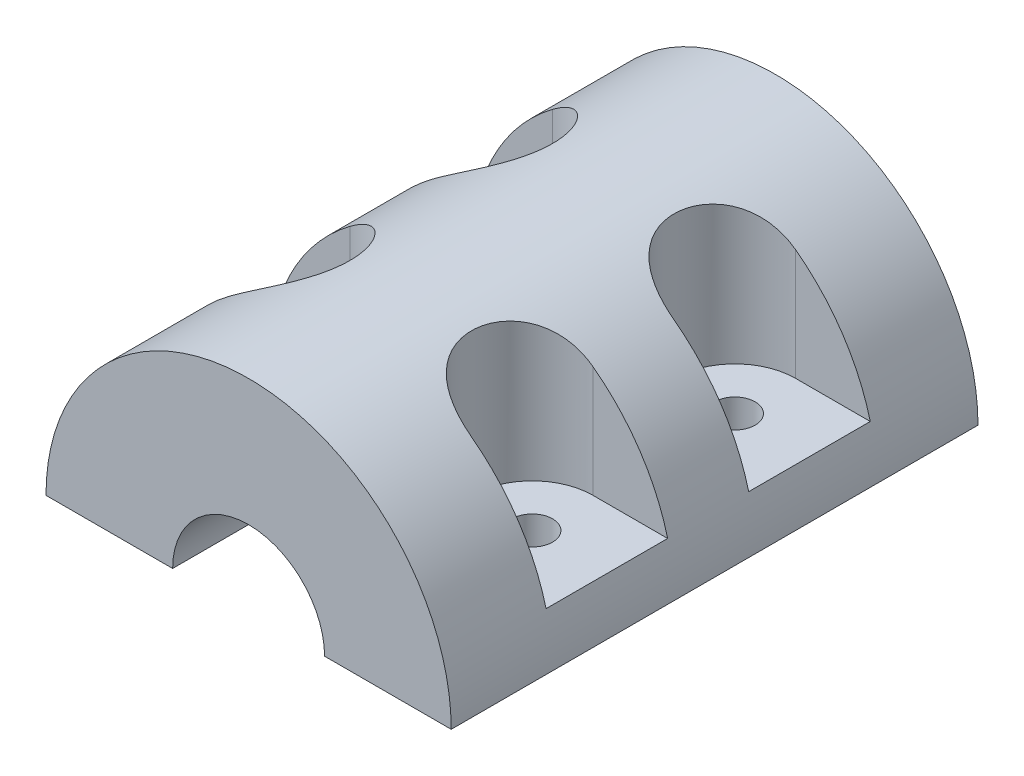
SolidWorks part; units mm, degrees
material "Plain Carbon Steel"
ref_plane "Front Plane" through (0, 0, 0) normal (0, 0, 1) x (1, 0, 0)
ref_plane "Top Plane" through (0, 0, 0) normal (0, 1, 0) x (1, 0, 0)
ref_plane "Right Plane" through (0, 0, 0) normal (1, 0, 0) x (0, 0, -1)
sketch "Block Profile Sketch" plane through (0, 0, 0) normal (0, 0, 1) x (1, 0, 0)
  line L0 (-100, 0) -> (-37.5, 0)
  line L1 (37.5, 0) -> (100, 0)
  arc A0 (100, 0) -> (-100, 0) centre (0, 0) ccw
  arc A1 (37.5, 0) -> (-37.5, 0) centre (0, 0) ccw
  dimension "D1" = 200
  dimension "D2" = 75
extrude "Block Body 260" add sketch "Block Profile Sketch" along normal mid plane 260
sketch "Bolt Pocket Sketch" plane through (0, 0, 0) normal (0, 1, 0) x (1, 0, 0)
  line L0 (-60, -20) -> (-100, -20)
  line L1 (-100, -20) -> (-100, -80)
  line L2 (-100, -80) -> (-60, -80)
  line L3 (-100, -130) -> (100, -130) construction
  line L4 (-100, -130) -> (-100, 130) construction
  arc A0 (-60, -80) -> (-60, -20) centre (-60, -50) ccw
  dimension "D1" = 60
  dimension "D2" = 80
  dimension "D4" = 40
extrude "Bolt Pocket 60x80" cut sketch "Bolt Pocket Sketch" along normal blind 260 from offset 25
mirror "Bolt Pocket Mirror Front" about plane through (0, 0, 0) normal (0, 0, 1) of "Bolt Pocket 60x80"
mirror "Bolt Pocket Mirror Right" about plane through (0, 0, 0) normal (1, 0, 0) of "Bolt Pocket Mirror Front", "Bolt Pocket 60x80"
sketch "Bolt Hole Sketch" plane through (0, 25, 0) normal (0, 1, 0) x (1, 0, 0)
  line L0 (-60, -80) -> (-60, -20) construction
  circle A0 centre (-60, -50) radius 10
  arc A1 (-60, -80) -> (-60, -20) centre (-60, -50) ccw construction
  dimension "D1" = 20
extrude "Bolt Hole Cut" cut sketch "Bolt Hole Sketch" against normal blind 260
mirror "Bolt Hole Mirror Front" about plane through (0, 0, 0) normal (0, 0, 1) of "Bolt Hole Cut"
mirror "Bolt Hole Mirror Right" about plane through (0, 0, 0) normal (1, 0, 0) of "Bolt Hole Mirror Front", "Bolt Hole Cut"
